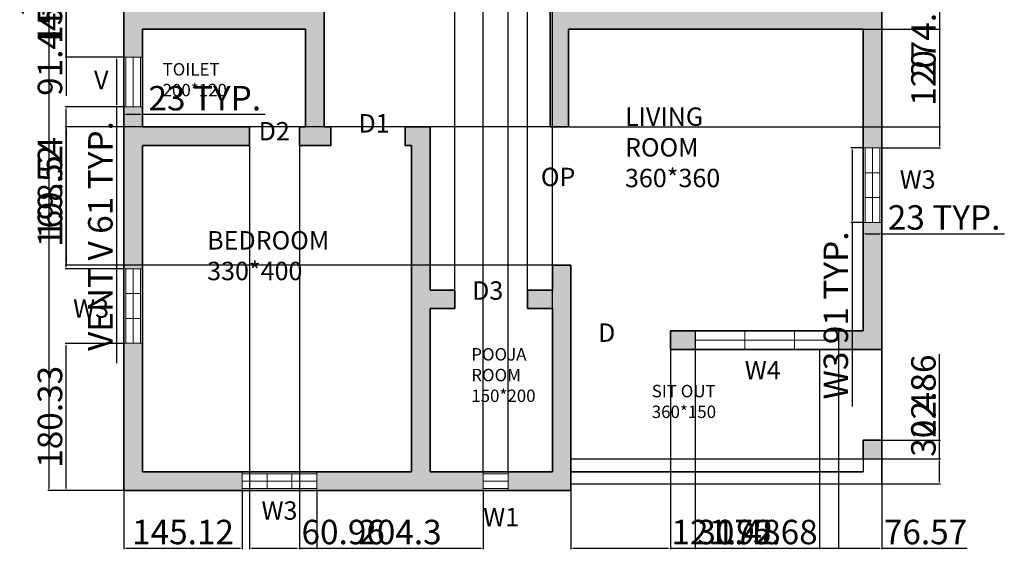
# Model space of a CAD drawing. Units: centimetres. Extents: x 2091 to 3299, y 1401 to 2845.
# Tile 1 of 2: x 2091 to 3299, y 1401 to 2053. Entities that reach past the tile are written whole.
import ezdxf

# ---------------------------------------------------------------- set-up
doc = ezdxf.new("R2010")
doc.units = ezdxf.units.CM
for name, color, linetype, lineweight in [('A-ANNO-DIMS', 2, 'Continuous', 18), ('A-ANNO-TEXT', 7, 'Continuous', 18), ('A-AREA-IDEN', 7, 'Continuous', 25), ('A-FLOR-STRS', 7, 'Continuous', 25), ('A-GLAZ', 4, 'Continuous', 18), ('A-WALL', 7, 'Continuous', 35)]:
    doc.layers.add(name, color=color, linetype=linetype, lineweight=lineweight)
doc.layers.add('A-WALL-PATT', color=18, linetype='Continuous', lineweight=13, true_color=0x000000)
doc.styles.get("Standard").update_dxf_attribs({"font": 'arial.ttf'})
doc.dimstyles.new('ISO-25', dxfattribs={"dimtxt": 30, "dimasz": 2.5, "dimexe": 1.25, "dimexo": 0.625, "dimtad": 1, "dimtxsty": 'Standard', "dimcen": 2.5, "dimadec": 0, "dimazin": 0, "dimtfac": 1, "dimtmove": 0, "dimatfit": 3, "dimfxl": 1, "dimarcsym": 0})

# ---------------------------------------------------------------- blocks, each defined once
blk = doc.blocks.new('*D2')
at = {"layer": 'A-ANNO-DIMS', "color": 0, "lineweight": -2, "transparency": 16777216}
for p, q in [((2218.2, 2725.5), (2125.3, 2725.5)), ((2126.6, 2723), (2126.6, 1478)), ((2218.2, 1475.5), (2125.3, 1475.5))]:
    blk.add_line(p, q, dxfattribs=at)
at = {"layer": 'A-ANNO-DIMS', "color": 0, "transparency": 16777216}
for points in [[(2126.2, 2723), (2127, 2723), (2126.6, 2725.5)], [(2126.2, 1478), (2127, 1478), (2126.6, 1475.5)]]:
    blk.add_solid(points, dxfattribs=at)
at = {"layer": 'Defpoints', "color": 0, "transparency": 16777216}
for p in [(2218.9, 2725.5), (2126.6, 1475.5), (2218.9, 1475.5)]:
    blk.add_point(p, dxfattribs=at)
at = {"layer": 'A-ANNO-DIMS', "color": 0, "transparency": 16777216, "insert": (2110.6, 2100.5), "char_height": 30, "attachment_point": 5, "rotation": 90}
blk.add_mtext('1250', dxfattribs=at)
blk = doc.blocks.new('WIN-W3')
for p, q in [((0, 0), (0, 22.9)), ((0, 20.3), (91.4, 20.3)), ((30.5, 2.5), (30.5, 20.3)), ((61, 2.5), (61, 20.3)), ((91.4, 22.9), (91.4, 0)), ((0, 11.4), (91.4, 11.4)), ((91.4, 2.5), (0, 2.5))]:
    blk.add_line(p, q)
blk = doc.blocks.new('VENT-V')
for p, q in [((0, 0), (0, 22.9)), ((0, 20.3), (61, 20.3)), ((61, 22.9), (61, 0)), ((0, 11.4), (61, 11.4)), ((61, 2.5), (0, 2.5))]:
    blk.add_line(p, q)
blk = doc.blocks.new('*D5')
at = {"layer": 'A-ANNO-DIMS', "color": 0, "lineweight": -2, "transparency": 16777216}
for p, q in [((3125.4, 1895.5), (3111, 1895.5)), ((3112.3, 1893), (3112.3, 1806.5)), ((3125.4, 1804), (3111, 1804)), ((3112.3, 1804), (3112.3, 1578.5))]:
    blk.add_line(p, q, dxfattribs=at)
at = {"layer": 'A-ANNO-DIMS', "color": 0, "transparency": 16777216}
for points in [[(3111.9, 1893), (3112.7, 1893), (3112.3, 1895.5)], [(3111.9, 1806.5), (3112.7, 1806.5), (3112.3, 1804)]]:
    blk.add_solid(points, dxfattribs=at)
at = {"layer": 'Defpoints', "color": 0, "transparency": 16777216}
for p in [(3126, 1895.5), (3112.3, 1804), (3126, 1804)]:
    blk.add_point(p, dxfattribs=at)
at = {"layer": 'A-ANNO-DIMS', "color": 0, "transparency": 16777216, "insert": (3096.3, 1690), "char_height": 30, "attachment_point": 5, "rotation": 90}
blk.add_mtext('W3 91 TYP.', dxfattribs=at)
blk = doc.blocks.new('*D6')
at = {"layer": 'A-ANNO-DIMS', "color": 0, "lineweight": -2, "transparency": 16777216}
for p, q in [((3126, 1803.4), (3126, 1789.1)), ((3148.9, 1803.4), (3148.9, 1789.1)), ((3128.5, 1790.3), (3146.4, 1790.3)), ((3148.9, 1790.3), (3299.2, 1790.3))]:
    blk.add_line(p, q, dxfattribs=at)
at = {"layer": 'A-ANNO-DIMS', "color": 0, "transparency": 16777216}
for points in [[(3128.5, 1790.7), (3128.5, 1789.9), (3126, 1790.3)], [(3146.4, 1790.7), (3146.4, 1789.9), (3148.9, 1790.3)]]:
    blk.add_solid(points, dxfattribs=at)
at = {"layer": 'Defpoints', "color": 0, "transparency": 16777216}
for p in [(3126, 1804), (3148.9, 1804), (3148.9, 1790.3)]:
    blk.add_point(p, dxfattribs=at)
at = {"layer": 'A-ANNO-DIMS', "color": 0, "transparency": 16777216, "insert": (3225.3, 1806.3), "char_height": 30, "attachment_point": 5}
blk.add_mtext('23 TYP.', dxfattribs=at)
blk = doc.blocks.new('*D7')
at = {"layer": 'A-ANNO-DIMS', "color": 0, "lineweight": -2, "transparency": 16777216}
for p, q in [((2218.2, 2006.8), (2208.5, 2006.8)), ((2209.7, 2004.3), (2209.7, 1948.3)), ((2218.2, 1945.8), (2208.5, 1945.8)), ((2209.7, 1945.8), (2209.7, 1631.5))]:
    blk.add_line(p, q, dxfattribs=at)
at = {"layer": 'A-ANNO-DIMS', "color": 0, "transparency": 16777216}
for points in [[(2209.3, 2004.3), (2210.1, 2004.3), (2209.7, 2006.8)], [(2209.3, 1948.3), (2210.1, 1948.3), (2209.7, 1945.8)]]:
    blk.add_solid(points, dxfattribs=at)
at = {"layer": 'Defpoints', "color": 0, "transparency": 16777216}
for p in [(2218.9, 2006.8), (2209.7, 1945.8), (2218.9, 1945.8)]:
    blk.add_point(p, dxfattribs=at)
at = {"layer": 'A-ANNO-DIMS', "color": 0, "transparency": 16777216, "insert": (2193.8, 1787.4), "char_height": 30, "attachment_point": 5, "rotation": 90}
blk.add_mtext('VENT V 61 TYP.', dxfattribs=at)
blk = doc.blocks.new('*D8')
at = {"layer": 'A-ANNO-DIMS', "color": 0, "lineweight": -2, "transparency": 16777216}
for p, q in [((2218.9, 1945.2), (2218.9, 1935.4)), ((2221.4, 1936.7), (2239.2, 1936.7)), ((2241.7, 1945.2), (2241.7, 1935.4)), ((2241.7, 1936.7), (2392, 1936.7))]:
    blk.add_line(p, q, dxfattribs=at)
at = {"layer": 'A-ANNO-DIMS', "color": 0, "transparency": 16777216}
for points in [[(2221.4, 1937.1), (2221.4, 1936.3), (2218.9, 1936.7)], [(2239.2, 1937.1), (2239.2, 1936.3), (2241.7, 1936.7)]]:
    blk.add_solid(points, dxfattribs=at)
at = {"layer": 'Defpoints', "color": 0, "transparency": 16777216}
for p in [(2218.9, 1945.8), (2241.7, 1945.8), (2241.7, 1936.7)]:
    blk.add_point(p, dxfattribs=at)
at = {"layer": 'A-ANNO-DIMS', "color": 0, "transparency": 16777216, "insert": (2318.1, 1952.6), "char_height": 30, "attachment_point": 5}
blk.add_mtext('23 TYP.', dxfattribs=at)
blk = doc.blocks.new('*D11')
at = {"layer": 'A-ANNO-DIMS', "color": 0, "lineweight": -2, "transparency": 16777216}
for p, q in [((2373.1, 1897.7), (2373.1, 1403.4)), ((2434.1, 1897.7), (2434.1, 1403.4)), ((2375.6, 1404.6), (2431.6, 1404.6)), ((2434.1, 1404.6), (2539.2, 1404.6))]:
    blk.add_line(p, q, dxfattribs=at)
at = {"layer": 'A-ANNO-DIMS', "color": 0, "transparency": 16777216}
for points in [[(2375.6, 1405), (2375.6, 1404.2), (2373.1, 1404.6)], [(2431.6, 1405), (2431.6, 1404.2), (2434.1, 1404.6)]]:
    blk.add_solid(points, dxfattribs=at)
at = {"layer": 'Defpoints', "color": 0, "transparency": 16777216}
for p in [(2373.1, 1898.4), (2434.1, 1898.4), (2434.1, 1404.6)]:
    blk.add_point(p, dxfattribs=at)
at = {"layer": 'A-ANNO-DIMS', "color": 0, "transparency": 16777216, "insert": (2487.9, 1420.6), "char_height": 30, "attachment_point": 5}
blk.add_mtext('60.96', dxfattribs=at)
blk = doc.blocks.new('*D12')
at = {"layer": 'A-ANNO-DIMS', "color": 0, "lineweight": -2, "transparency": 16777216}
for p, q in [((2625.1, 1721.9), (2625.1, 2797.7)), ((2627.6, 2796.4), (2711.6, 2796.4)), ((2714.1, 1721.9), (2714.1, 2797.7)), ((2714.1, 2796.4), (2819, 2796.4))]:
    blk.add_line(p, q, dxfattribs=at)
at = {"layer": 'A-ANNO-DIMS', "color": 0, "transparency": 16777216}
for points in [[(2627.6, 2796.8), (2627.6, 2796), (2625.1, 2796.4)], [(2711.6, 2796.8), (2711.6, 2796), (2714.1, 2796.4)]]:
    blk.add_solid(points, dxfattribs=at)
at = {"layer": 'Defpoints', "color": 0, "transparency": 16777216}
for p in [(2714.1, 2796.4), (2625.1, 1721.2), (2714.1, 1721.2)]:
    blk.add_point(p, dxfattribs=at)
at = {"layer": 'A-ANNO-DIMS', "color": 0, "transparency": 16777216, "insert": (2767.8, 2812.4), "char_height": 30, "attachment_point": 5}
blk.add_mtext('89.04', dxfattribs=at)
blk = doc.blocks.new('*D13')
at = {"layer": 'A-ANNO-DIMS', "color": 0, "lineweight": -2, "transparency": 16777216}
for p, q in [((2714.1, 1699), (2714.1, 2797.7)), ((2716.6, 2796.4), (2742.1, 2796.4)), ((2744.6, 1699), (2744.6, 2797.7)), ((2744.6, 2796.4), (2849.6, 2796.4))]:
    blk.add_line(p, q, dxfattribs=at)
at = {"layer": 'A-ANNO-DIMS', "color": 0, "transparency": 16777216}
for points in [[(2716.6, 2796.8), (2716.6, 2796), (2714.1, 2796.4)], [(2742.1, 2796.8), (2742.1, 2796), (2744.6, 2796.4)]]:
    blk.add_solid(points, dxfattribs=at)
at = {"layer": 'Defpoints', "color": 0, "transparency": 16777216}
for p in [(2744.6, 2796.4), (2714.1, 1698.4), (2744.6, 1698.4)]:
    blk.add_point(p, dxfattribs=at)
at = {"layer": 'A-ANNO-DIMS', "color": 0, "transparency": 16777216, "insert": (2798.3, 2812.4), "char_height": 30, "attachment_point": 5}
blk.add_mtext('30.48', dxfattribs=at)
blk = doc.blocks.new('*D14')
at = {"layer": 'A-ANNO-DIMS', "color": 0, "lineweight": -2, "transparency": 16777216}
for p, q in [((2741.1, 1921.2), (2146.7, 1921.2)), ((2148, 1918.7), (2148, 1754.2)), ((2744, 1751.7), (2146.7, 1751.7))]:
    blk.add_line(p, q, dxfattribs=at)
at = {"layer": 'A-ANNO-DIMS', "color": 0, "transparency": 16777216}
for points in [[(2147.5, 1918.7), (2148.4, 1918.7), (2148, 1921.2)], [(2147.5, 1754.2), (2148.4, 1754.2), (2148, 1751.7)]]:
    blk.add_solid(points, dxfattribs=at)
at = {"layer": 'Defpoints', "color": 0, "transparency": 16777216}
for p in [(2741.7, 1921.2), (2148, 1751.7), (2744.6, 1751.7)]:
    blk.add_point(p, dxfattribs=at)
at = {"layer": 'A-ANNO-DIMS', "color": 0, "transparency": 16777216, "insert": (2132, 1836.5), "char_height": 30, "attachment_point": 5, "rotation": 90}
blk.add_mtext('169.52', dxfattribs=at)
blk = doc.blocks.new('*D15')
at = {"layer": 'A-ANNO-DIMS', "color": 0, "lineweight": -2, "transparency": 16777216}
for p, q in [((2765.2, 2041.2), (3221, 2041.2)), ((3219.8, 2038.7), (3219.8, 1923.7)), ((2765.2, 1921.2), (3221, 1921.2))]:
    blk.add_line(p, q, dxfattribs=at)
at = {"layer": 'A-ANNO-DIMS', "color": 0, "transparency": 16777216}
for points in [[(3219.3, 2038.7), (3220.2, 2038.7), (3219.8, 2041.2)], [(3219.3, 1923.7), (3220.2, 1923.7), (3219.8, 1921.2)]]:
    blk.add_solid(points, dxfattribs=at)
at = {"layer": 'Defpoints', "color": 0, "transparency": 16777216}
for p in [(2764.6, 2041.2), (2764.6, 1921.2), (3219.8, 1921.2)]:
    blk.add_point(p, dxfattribs=at)
at = {"layer": 'A-ANNO-DIMS', "color": 0, "transparency": 16777216, "insert": (3203.8, 1981.2), "char_height": 30, "attachment_point": 5, "rotation": 90}
blk.add_mtext('120', dxfattribs=at)
blk = doc.blocks.new('*D16')
at = {"layer": 'A-ANNO-DIMS', "color": 0, "lineweight": -2, "transparency": 16777216}
for p, q in [((2767.4, 1751.1), (2767.4, 1403.4)), ((2889.4, 1670.6), (2889.4, 1403.4)), ((2769.9, 1404.6), (2886.9, 1404.6)), ((2889.4, 1404.6), (3014.5, 1404.6))]:
    blk.add_line(p, q, dxfattribs=at)
at = {"layer": 'A-ANNO-DIMS', "color": 0, "transparency": 16777216}
for points in [[(2769.9, 1405), (2769.9, 1404.2), (2767.4, 1404.6)], [(2886.9, 1405), (2886.9, 1404.2), (2889.4, 1404.6)]]:
    blk.add_solid(points, dxfattribs=at)
at = {"layer": 'Defpoints', "color": 0, "transparency": 16777216}
for p in [(2767.4, 1751.7), (2889.4, 1671.2), (2889.4, 1404.6)]:
    blk.add_point(p, dxfattribs=at)
at = {"layer": 'A-ANNO-DIMS', "color": 0, "transparency": 16777216, "insert": (2953.2, 1420.6), "char_height": 30, "attachment_point": 5}
blk.add_mtext('121.92', dxfattribs=at)
blk = doc.blocks.new('*D17')
at = {"layer": 'A-ANNO-DIMS', "color": 0, "lineweight": -2, "transparency": 16777216}
for p, q in [((2919.8, 1670.6), (2919.8, 1403.4)), ((3095.5, 1670.6), (3095.5, 1403.4)), ((2922.3, 1404.6), (3093, 1404.6))]:
    blk.add_line(p, q, dxfattribs=at)
at = {"layer": 'A-ANNO-DIMS', "color": 0, "transparency": 16777216}
for points in [[(2922.3, 1405), (2922.3, 1404.2), (2919.8, 1404.6)], [(3093, 1405), (3093, 1404.2), (3095.5, 1404.6)]]:
    blk.add_solid(points, dxfattribs=at)
at = {"layer": 'Defpoints', "color": 0, "transparency": 16777216}
for p in [(2919.8, 1671.2), (3095.5, 1671.2), (3095.5, 1404.6)]:
    blk.add_point(p, dxfattribs=at)
at = {"layer": 'A-ANNO-DIMS', "color": 0, "transparency": 16777216, "insert": (3007.7, 1420.6), "char_height": 30, "attachment_point": 5}
blk.add_mtext('175.68', dxfattribs=at)
blk = doc.blocks.new('*D18')
at = {"layer": 'A-ANNO-DIMS', "color": 0, "lineweight": -2, "transparency": 16777216}
for p, q in [((2889.4, 1647.7), (2889.4, 1403.4)), ((2919.8, 1647.7), (2919.8, 1403.4)), ((2891.9, 1404.6), (2917.3, 1404.6)), ((2919.8, 1404.6), (3024.9, 1404.6))]:
    blk.add_line(p, q, dxfattribs=at)
at = {"layer": 'A-ANNO-DIMS', "color": 0, "transparency": 16777216}
for points in [[(2891.9, 1405), (2891.9, 1404.2), (2889.4, 1404.6)], [(2917.3, 1405), (2917.3, 1404.2), (2919.8, 1404.6)]]:
    blk.add_solid(points, dxfattribs=at)
at = {"layer": 'Defpoints', "color": 0, "transparency": 16777216}
for p in [(2889.4, 1648.4), (2919.8, 1648.4), (2919.8, 1404.6)]:
    blk.add_point(p, dxfattribs=at)
at = {"layer": 'A-ANNO-DIMS', "color": 0, "transparency": 16777216, "insert": (2973.6, 1420.6), "char_height": 30, "attachment_point": 5}
blk.add_mtext('30.48', dxfattribs=at)
blk = doc.blocks.new('*D21')
at = {"layer": 'A-ANNO-DIMS', "color": 0, "lineweight": -2, "transparency": 16777216}
for p, q in [((2241.1, 2155.5), (2146.7, 2155.5)), ((2148, 2153), (2148, 2066.6)), ((2241.1, 2064.1), (2146.7, 2064.1)), ((2148, 2064.1), (2148, 1959.2))]:
    blk.add_line(p, q, dxfattribs=at)
at = {"layer": 'A-ANNO-DIMS', "color": 0, "transparency": 16777216}
for points in [[(2147.5, 2153), (2148.4, 2153), (2148, 2155.5)], [(2147.5, 2066.6), (2148.4, 2066.6), (2148, 2064.1)]]:
    blk.add_solid(points, dxfattribs=at)
at = {"layer": 'Defpoints', "color": 0, "transparency": 16777216}
for p in [(2241.7, 2155.5), (2148, 2064.1), (2241.7, 2064.1)]:
    blk.add_point(p, dxfattribs=at)
at = {"layer": 'A-ANNO-DIMS', "color": 0, "transparency": 16777216, "insert": (2132, 2010.4), "char_height": 30, "attachment_point": 5, "rotation": 90}
blk.add_mtext('91.44', dxfattribs=at)
blk = doc.blocks.new('*D22')
at = {"layer": 'A-ANNO-DIMS', "color": 0, "lineweight": -2, "transparency": 16777216}
for p, q in [((2218.9, 1474.9), (2218.9, 1403.4)), ((2364, 1474.9), (2364, 1403.4)), ((2221.4, 1404.6), (2361.5, 1404.6))]:
    blk.add_line(p, q, dxfattribs=at)
at = {"layer": 'A-ANNO-DIMS', "color": 0, "transparency": 16777216}
for points in [[(2221.4, 1405), (2221.4, 1404.2), (2218.9, 1404.6)], [(2361.5, 1405), (2361.5, 1404.2), (2364, 1404.6)]]:
    blk.add_solid(points, dxfattribs=at)
at = {"layer": 'Defpoints', "color": 0, "transparency": 16777216}
for p in [(2218.9, 1475.5), (2364, 1475.5), (2364, 1404.6)]:
    blk.add_point(p, dxfattribs=at)
at = {"layer": 'A-ANNO-DIMS', "color": 0, "transparency": 16777216, "insert": (2291.4, 1420.6), "char_height": 30, "attachment_point": 5}
blk.add_mtext('145.12', dxfattribs=at)
blk = doc.blocks.new('*D23')
at = {"layer": 'A-ANNO-DIMS', "color": 0, "lineweight": -2, "transparency": 16777216}
for p, q in [((2455.4, 1474.9), (2455.4, 1403.4)), ((2659.7, 1474.9), (2659.7, 1403.4)), ((2457.9, 1404.6), (2657.2, 1404.6))]:
    blk.add_line(p, q, dxfattribs=at)
at = {"layer": 'A-ANNO-DIMS', "color": 0, "transparency": 16777216}
for points in [[(2457.9, 1405), (2457.9, 1404.2), (2455.4, 1404.6)], [(2657.2, 1405), (2657.2, 1404.2), (2659.7, 1404.6)]]:
    blk.add_solid(points, dxfattribs=at)
at = {"layer": 'Defpoints', "color": 0, "transparency": 16777216}
for p in [(2455.4, 1475.5), (2659.7, 1475.5), (2659.7, 1404.6)]:
    blk.add_point(p, dxfattribs=at)
at = {"layer": 'A-ANNO-DIMS', "color": 0, "transparency": 16777216, "insert": (2557.6, 1420.6), "char_height": 30, "attachment_point": 5}
blk.add_mtext('204.3', dxfattribs=at)
blk = doc.blocks.new('*D24')
at = {"layer": 'A-ANNO-DIMS', "color": 0, "lineweight": -2, "transparency": 16777216}
for p, q in [((2659.7, 1499), (2659.7, 2797.7)), ((2662.2, 2796.4), (2687.7, 2796.4)), ((2690.2, 1499), (2690.2, 2797.7)), ((2690.2, 2796.4), (2795.2, 2796.4))]:
    blk.add_line(p, q, dxfattribs=at)
at = {"layer": 'A-ANNO-DIMS', "color": 0, "transparency": 16777216}
for points in [[(2662.2, 2796.8), (2662.2, 2796), (2659.7, 2796.4)], [(2687.7, 2796.8), (2687.7, 2796), (2690.2, 2796.4)]]:
    blk.add_solid(points, dxfattribs=at)
at = {"layer": 'Defpoints', "color": 0, "transparency": 16777216}
for p in [(2690.2, 2796.4), (2659.7, 1498.4), (2690.2, 1498.4)]:
    blk.add_point(p, dxfattribs=at)
at = {"layer": 'A-ANNO-DIMS', "color": 0, "transparency": 16777216, "insert": (2744, 2812.4), "char_height": 30, "attachment_point": 5}
blk.add_mtext('30.48', dxfattribs=at)
blk = doc.blocks.new('*D25')
at = {"layer": 'A-ANNO-DIMS', "color": 0, "lineweight": -2, "transparency": 16777216}
for p, q in [((2218.2, 1655.8), (2146.7, 1655.8)), ((2148, 1478), (2148, 1653.3)), ((2218.2, 1475.5), (2146.7, 1475.5))]:
    blk.add_line(p, q, dxfattribs=at)
at = {"layer": 'A-ANNO-DIMS', "color": 0, "transparency": 16777216}
for points in [[(2147.5, 1653.3), (2148.4, 1653.3), (2148, 1655.8)], [(2147.5, 1478), (2148.4, 1478), (2148, 1475.5)]]:
    blk.add_solid(points, dxfattribs=at)
at = {"layer": 'Defpoints', "color": 0, "transparency": 16777216}
for p in [(2148, 1655.8), (2218.9, 1655.8), (2218.9, 1475.5)]:
    blk.add_point(p, dxfattribs=at)
at = {"layer": 'A-ANNO-DIMS', "color": 0, "transparency": 16777216, "insert": (2132, 1565.7), "char_height": 30, "attachment_point": 5, "rotation": 90}
blk.add_mtext('180.33', dxfattribs=at)
blk = doc.blocks.new('*D26')
at = {"layer": 'A-ANNO-DIMS', "color": 0, "lineweight": -2, "transparency": 16777216}
for p, q in [((2218.2, 1945.8), (2146.7, 1945.8)), ((2148, 1749.8), (2148, 1943.3)), ((2218.2, 1747.3), (2146.7, 1747.3))]:
    blk.add_line(p, q, dxfattribs=at)
at = {"layer": 'A-ANNO-DIMS', "color": 0, "transparency": 16777216}
for points in [[(2147.5, 1943.3), (2148.4, 1943.3), (2148, 1945.8)], [(2147.5, 1749.8), (2148.4, 1749.8), (2148, 1747.3)]]:
    blk.add_solid(points, dxfattribs=at)
at = {"layer": 'Defpoints', "color": 0, "transparency": 16777216}
for p in [(2148, 1945.8), (2218.9, 1945.8), (2218.9, 1747.3)]:
    blk.add_point(p, dxfattribs=at)
at = {"layer": 'A-ANNO-DIMS', "color": 0, "transparency": 16777216, "insert": (2132, 1846.6), "char_height": 30, "attachment_point": 5, "rotation": 90}
blk.add_mtext('198.54', dxfattribs=at)
blk = doc.blocks.new('*D27')
at = {"layer": 'A-ANNO-DIMS', "color": 0, "lineweight": -2, "transparency": 16777216}
for p, q in [((2218.2, 2164.2), (2146.7, 2164.2)), ((2148, 2009.3), (2148, 2161.7)), ((2218.2, 2006.8), (2146.7, 2006.8))]:
    blk.add_line(p, q, dxfattribs=at)
at = {"layer": 'A-ANNO-DIMS', "color": 0, "transparency": 16777216}
for points in [[(2147.5, 2161.7), (2148.4, 2161.7), (2148, 2164.2)], [(2147.5, 2009.3), (2148.4, 2009.3), (2148, 2006.8)]]:
    blk.add_solid(points, dxfattribs=at)
at = {"layer": 'Defpoints', "color": 0, "transparency": 16777216}
for p in [(2148, 2164.2), (2218.9, 2164.2), (2218.9, 2006.8)]:
    blk.add_point(p, dxfattribs=at)
at = {"layer": 'A-ANNO-DIMS', "color": 0, "transparency": 16777216, "insert": (2132, 2085.5), "char_height": 30, "attachment_point": 5, "rotation": 90}
blk.add_mtext('157.44', dxfattribs=at)
blk = doc.blocks.new('*D33')
at = {"layer": 'A-ANNO-DIMS', "color": 0, "lineweight": -2, "transparency": 16777216}
for p, q in [((3149.5, 2169.8), (3221, 2169.8)), ((3219.8, 2167.3), (3219.8, 1898)), ((3149.5, 1895.5), (3221, 1895.5))]:
    blk.add_line(p, q, dxfattribs=at)
at = {"layer": 'A-ANNO-DIMS', "color": 0, "transparency": 16777216}
for points in [[(3219.3, 2167.3), (3220.2, 2167.3), (3219.8, 2169.8)], [(3219.3, 1898), (3220.2, 1898), (3219.8, 1895.5)]]:
    blk.add_solid(points, dxfattribs=at)
at = {"layer": 'Defpoints', "color": 0, "transparency": 16777216}
for p in [(3148.9, 2169.8), (3148.9, 1895.5), (3219.8, 1895.5)]:
    blk.add_point(p, dxfattribs=at)
at = {"layer": 'A-ANNO-DIMS', "color": 0, "transparency": 16777216, "insert": (3203.8, 2032.6), "char_height": 30, "attachment_point": 5, "rotation": 90}
blk.add_mtext('274.3', dxfattribs=at)
blk = doc.blocks.new('*D34')
at = {"layer": 'A-ANNO-DIMS', "color": 0, "lineweight": -2, "transparency": 16777216}
for p, q in [((3072.3, 1513.5), (3072.3, 1403.4)), ((3148.9, 1513.5), (3148.9, 1403.4)), ((3074.8, 1404.6), (3146.4, 1404.6)), ((3148.9, 1404.6), (3253.6, 1404.6))]:
    blk.add_line(p, q, dxfattribs=at)
at = {"layer": 'A-ANNO-DIMS', "color": 0, "transparency": 16777216}
for points in [[(3074.8, 1405), (3074.8, 1404.2), (3072.3, 1404.6)], [(3146.4, 1405), (3146.4, 1404.2), (3148.9, 1404.6)]]:
    blk.add_solid(points, dxfattribs=at)
at = {"layer": 'Defpoints', "color": 0, "transparency": 16777216}
for p in [(3072.3, 1514.1), (3148.9, 1514.1), (3148.9, 1404.6)]:
    blk.add_point(p, dxfattribs=at)
at = {"layer": 'A-ANNO-DIMS', "color": 0, "transparency": 16777216, "insert": (3202.5, 1420.6), "char_height": 30, "attachment_point": 5}
blk.add_mtext('76.57', dxfattribs=at)
blk = doc.blocks.new('*D35')
at = {"layer": 'A-ANNO-DIMS', "color": 0, "lineweight": -2, "transparency": 16777216}
for p, q in [((3219.8, 1514.1), (3219.8, 1619.1)), ((3149.5, 1514.1), (3221, 1514.1)), ((3219.8, 1486.1), (3219.8, 1511.6)), ((3149.5, 1483.6), (3221, 1483.6))]:
    blk.add_line(p, q, dxfattribs=at)
at = {"layer": 'A-ANNO-DIMS', "color": 0, "transparency": 16777216}
for points in [[(3219.3, 1511.6), (3220.2, 1511.6), (3219.8, 1514.1)], [(3219.3, 1486.1), (3220.2, 1486.1), (3219.8, 1483.6)]]:
    blk.add_solid(points, dxfattribs=at)
at = {"layer": 'Defpoints', "color": 0, "transparency": 16777216}
for p in [(3148.9, 1514.1), (3219.8, 1514.1), (3148.9, 1483.6)]:
    blk.add_point(p, dxfattribs=at)
at = {"layer": 'A-ANNO-DIMS', "color": 0, "transparency": 16777216, "insert": (3203.8, 1567.9), "char_height": 30, "attachment_point": 5, "rotation": 90}
blk.add_mtext('30.48', dxfattribs=at)
blk = doc.blocks.new('*D36')
at = {"layer": 'A-ANNO-DIMS', "color": 0, "lineweight": -2, "transparency": 16777216}
for p, q in [((3219.8, 1537), (3219.8, 1642.4)), ((3149.5, 1537), (3221, 1537)), ((3219.8, 1516.6), (3219.8, 1534.5)), ((3149.5, 1514.1), (3221, 1514.1))]:
    blk.add_line(p, q, dxfattribs=at)
at = {"layer": 'A-ANNO-DIMS', "color": 0, "transparency": 16777216}
for points in [[(3219.3, 1534.5), (3220.2, 1534.5), (3219.8, 1537)], [(3219.3, 1516.6), (3220.2, 1516.6), (3219.8, 1514.1)]]:
    blk.add_solid(points, dxfattribs=at)
at = {"layer": 'Defpoints', "color": 0, "transparency": 16777216}
for p in [(3148.9, 1537), (3219.8, 1537), (3148.9, 1514.1)]:
    blk.add_point(p, dxfattribs=at)
at = {"layer": 'A-ANNO-DIMS', "color": 0, "transparency": 16777216, "insert": (3203.8, 1591), "char_height": 30, "attachment_point": 5, "rotation": 90}
blk.add_mtext('22.86', dxfattribs=at)

msp = doc.modelspace()

# ---------------------------------------------------------------- hatches: boundary and pattern name
at = {"layer": 'A-WALL-PATT'}
h = msp.add_hatch(color=256, dxfattribs=at)
h.dxf.hatch_style = 1
h.paths.add_polyline_path([(2629.919, 2725.51), (2218.865, 2725.51), (2218.865, 2614.708), (2241.725, 2614.708), (2241.725, 2702.65), (2571.725, 2702.65), (2571.725, 2695.03), (2594.585, 2695.03), (2594.585, 2702.65), (2629.919, 2702.65)])
h.paths.add_polyline_path([(2902.29, 2725.51), (2690.879, 2725.51), (2690.879, 2702.65), (2714.585, 2702.65), (2714.585, 2522.65), (2594.585, 2522.65), (2594.585, 2634.77), (2571.725, 2634.77), (2571.725, 2386.95), (2564.105, 2386.95), (2564.105, 2364.09), (2602.205, 2364.09), (2602.205, 2386.95), (2594.585, 2386.95), (2594.585, 2499.79), (2737.445, 2499.79), (2737.445, 2702.65), (2902.29, 2702.65)])
h.paths.add_polyline_path([(3148.865, 2725.51), (2993.73, 2725.51), (2993.73, 2702.65), (3126.005, 2702.65), (3126.005, 2600.88), (3148.865, 2600.88)])
h.paths.add_polyline_path([(3148.865, 2509.44), (3126.005, 2509.44), (3126.005, 2386.95), (2693.645, 2386.95), (2693.645, 2364.09), (2741.725, 2364.09), (2741.725, 2356.47), (2764.585, 2356.47), (2764.585, 2364.09), (3126.005, 2364.09), (3126.005, 2261.228), (3148.865, 2261.228)])
h.paths.add_polyline_path([(2472.665, 2386.95), (2241.725, 2386.95), (2241.725, 2523.268), (2218.865, 2523.268), (2218.865, 2255.666), (2241.725, 2255.666), (2241.725, 2364.09), (2472.665, 2364.09)])
h.paths.add_polyline_path([(3148.865, 2169.788), (3126.005, 2169.788), (3126.005, 2064.09), (2764.585, 2064.09), (2764.585, 2265.03), (2741.725, 2265.03), (2741.725, 1921.23), (2764.585, 1921.23), (2764.585, 2041.23), (3126.005, 2041.23), (3126.005, 1895.472), (3148.865, 1895.472)])
h.paths.add_polyline_path([(3148.865, 1804.032), (3126.005, 1804.032), (3126.005, 1671.23), (3095.525, 1671.23), (3095.525, 1648.37), (3148.865, 1648.37)])
h.paths.add_polyline_path([(2241.725, 2155.53), (2241.725, 2164.226), (2218.865, 2164.226), (2218.865, 2006.784), (2241.725, 2006.784), (2241.725, 2041.23), (2441.725, 2041.23), (2441.725, 1921.23), (2434.105, 1921.23), (2434.105, 1898.37), (2472.665, 1898.37), (2472.665, 1921.23), (2464.585, 1921.23), (2464.585, 2064.09), (2241.725, 2064.09)])
h.paths.add_polyline_path([(2241.725, 1898.37), (2373.145, 1898.37), (2373.145, 1921.23), (2241.725, 1921.23), (2241.725, 1945.824), (2218.865, 1945.824), (2218.865, 1747.285), (2241.725, 1747.285)])
h.paths.add_polyline_path([(2241.725, 1655.845), (2218.865, 1655.845), (2218.865, 1475.51), (2363.981, 1475.51), (2363.981, 1498.37), (2241.725, 1498.37)])
h.paths.add_polyline_path([(2594.585, 1921.23), (2564.105, 1921.23), (2564.105, 1898.37), (2571.725, 1898.37), (2571.725, 1498.37), (2455.421, 1498.37), (2455.421, 1475.51), (2659.718, 1475.51), (2659.718, 1498.37), (2594.585, 1498.37), (2594.585, 1698.37), (2625.065, 1698.37), (2625.065, 1721.23), (2594.585, 1721.23)])
h.paths.add_polyline_path([(2767.445, 1721.23), (2767.445, 1751.71), (2744.585, 1751.71), (2744.585, 1721.23), (2714.105, 1721.23), (2714.105, 1698.37), (2744.585, 1698.37), (2744.585, 1498.37), (2690.198, 1498.37), (2690.198, 1475.51), (2767.445, 1475.51)])
h.paths.add_polyline_path([(3148.865, 1536.968), (3126.005, 1536.968), (3126.005, 1514.108), (3148.865, 1514.108)])
h.paths.add_polyline_path([(2919.845, 1671.23), (2889.365, 1671.23), (2889.365, 1648.37), (2919.845, 1648.37)])

# ---------------------------------------------------------------- linework, layer by layer
at = {"layer": 'A-FLOR-STRS'}
for p, q in [((3072.296, 1648.37), (3072.296, 1514.108)), ((2767.445, 1514.108), (3148.865, 1514.108)), ((3126.005, 1514.108), (3126.005, 1498.37)), ((3126.005, 1498.37), (2767.445, 1498.37)), ((2767.445, 1498.37), (3126.005, 1498.37)), ((2767.445, 1483.628), (3148.865, 1483.628))]:
    msp.add_line(p, q, dxfattribs=at)
at = {"layer": 'A-GLAZ'}
for p, q in [((2919.845, 1648.37), (2919.845, 1671.23)), ((2980.805, 1648.37), (2980.805, 1671.23)), ((3041.765, 1648.37), (3041.765, 1671.23)), ((3095.525, 1671.23), (3095.525, 1648.37)), ((2919.845, 1659.8), (3095.525, 1659.8)), ((2659.718, 1498.37), (2659.718, 1475.51)), ((2690.198, 1475.51), (2690.198, 1498.37)), ((2690.198, 1495.83), (2659.718, 1495.83)), ((2659.718, 1486.94), (2690.198, 1486.94)), ((2659.718, 1478.05), (2690.198, 1478.05))]:
    msp.add_line(p, q, dxfattribs=at)
at = {"layer": 'A-WALL'}
for p, q in [((2218.865, 1475.51), (2218.865, 2725.51)), ((3148.865, 2725.51), (3148.865, 1483.628)), ((2741.725, 1921.23), (2741.725, 2265.03)), ((2464.585, 2064.09), (2464.585, 1921.23)), ((2441.725, 2041.23), (2241.725, 2041.23)), ((2241.725, 1921.23), (2241.725, 2041.23)), ((2441.725, 2041.23), (2441.725, 1921.23)), ((3126.005, 2041.23), (2764.585, 2041.23)), ((2764.585, 1921.23), (2764.585, 2041.23)), ((3126.005, 2041.23), (3126.005, 1671.23)), ((2373.145, 1921.23), (2241.725, 1921.23)), ((2373.145, 1921.23), (2373.145, 1898.37)), ((2434.105, 1921.23), (2434.105, 1898.37)), ((2441.725, 1921.23), (2434.105, 1921.23)), ((2472.665, 1921.23), (2464.585, 1921.23)), ((2472.665, 1898.37), (2472.665, 1921.23)), ((2564.105, 1898.37), (2564.105, 1921.23)), ((2594.585, 1921.23), (2564.105, 1921.23)), ((2594.585, 1721.23), (2594.585, 1921.23)), ((2741.725, 1921.23), (2764.585, 1921.23)), ((2241.725, 1498.37), (2241.725, 1898.37)), ((2373.145, 1898.37), (2241.725, 1898.37)), ((2472.665, 1898.37), (2434.105, 1898.37)), ((2571.725, 1898.37), (2564.105, 1898.37)), ((2571.725, 1498.37), (2571.725, 1898.37)), ((2767.445, 1751.71), (2744.585, 1751.71)), ((2744.585, 1751.71), (2744.585, 1721.23)), ((2767.445, 1721.23), (2767.445, 1751.71)), ((2594.585, 1721.23), (2625.065, 1721.23)), ((2625.065, 1698.37), (2625.065, 1721.23)), ((2714.105, 1698.37), (2714.105, 1721.23)), ((2714.105, 1721.23), (2744.585, 1721.23)), ((2767.445, 1475.51), (2767.445, 1721.23)), ((2594.585, 1498.37), (2594.585, 1698.37)), ((2594.585, 1698.37), (2625.065, 1698.37)), ((2594.585, 1698.37), (2625.065, 1698.37)), ((2594.585, 1698.37), (2625.065, 1698.37)), ((2714.105, 1698.37), (2744.585, 1698.37)), ((2744.585, 1698.37), (2741.105, 1698.37)), ((2744.585, 1498.37), (2744.585, 1698.37)), ((2889.365, 1671.23), (3126.005, 1671.23)), ((2889.365, 1648.37), (2889.365, 1671.23)), ((2889.365, 1648.37), (3148.865, 1648.37)), ((3126.005, 1514.108), (3126.005, 1536.968)), ((3126.005, 1536.968), (3148.865, 1536.968)), ((2571.725, 1498.37), (2241.725, 1498.37)), ((2744.585, 1498.37), (2594.585, 1498.37)), ((2767.445, 1475.51), (2218.865, 1475.51))]:
    msp.add_line(p, q, dxfattribs=at)

# ---------------------------------------------------------------- block references
at = {"layer": 'A-GLAZ'}
for name, p, rotation in [('VENT-V', (2218.866, 2006.784), 269.9999999999984), ('WIN-W3', (3126.006, 1895.472), 270), ('WIN-W3', (2218.866, 1747.285), 270.0000000000006)]:
    msp.add_blockref(name, p, dxfattribs=dict(at, rotation=rotation))
msp.add_blockref('WIN-W3', (2363.981, 1475.51), dxfattribs=at)

# ---------------------------------------------------------------- texts
at = {"layer": 'A-ANNO-TEXT', "char_height": 22.56, "attachment_point": 1}
for s, width, insert in [('V', 39.89904, (2182.186, 1989.998)), ('D1', 21.81012, (2506.661, 1936.92)), ('D2', 22.59147, (2384.165, 1927.249)), ('OP', 36.39872, (2730.479, 1871.174)), ('W3', 162.65151, (3170.799, 1868.053)), ('D3', 40.55497, (2646.093, 1731.861)), ('W3', 162.65151, (2156.466, 1709.852)), ('D', 51.99818, (2800.676, 1680.233)), ('W4', 162.65151, (2980.628, 1634.308)), ('W3', 162.65151, (2387.643, 1462.118)), ('W1', 162.65151, (2659.718, 1454.126))]:
    msp.add_mtext_dynamic_manual_height_columns(s, width=width, gutter_width=12.5, heights=[0], dxfattribs=dict(at, insert=insert))
at = {"layer": 'A-AREA-IDEN', "attachment_point": 1}
for s, width, insert, char_height in [('TOILET\\P200*120', 85.88212, (2266.279, 1999.409), 15.24), ('LIVING ROOM\\P360*360', 166.11333, (2833.712, 1945.065), 22.56), ('BEDROOM\\P330*400', 184.57037, (2321.017, 1793.427), 22.56), ('POOJA ROOM \\P150*200', 65.62503, (2645.04, 1649.986), 15.24), ('SIT OUT \\P360*150', 92.28519, (2866.525, 1604.905), 15.24)]:
    msp.add_mtext_dynamic_manual_height_columns(s, width=width, gutter_width=12.5, heights=[0], dxfattribs=dict(at, insert=insert, char_height=char_height))

# ---------------------------------------------------------------- dimensions: what is measured, and where the dimension line sits
at = {"layer": 'A-ANNO-DIMS'}
for base, p1, p2, override, picture, middle in [((2714.105, 2796.41), (2625.065, 1721.23), (2714.105, 1721.23), {"dimdec": 2, "dimlfac": 1, "dimrnd": 0, "dimzin": 0, "dimdsep": 46, "dimlunit": 2}, '*D12', (2767.807, 2812.352)), ((2690.198, 2796.41), (2659.718, 1498.37), (2690.198, 1498.37), {"dimdec": 2, "dimlfac": 1, "dimrnd": 0, "dimzin": 0, "dimdsep": 46, "dimlunit": 2}, '*D24', (2743.961, 2812.362)), ((2744.585, 2796.41), (2714.105, 1698.37), (2744.585, 1698.37), {"dimdec": 2, "dimlfac": 1, "dimrnd": 0, "dimzin": 0, "dimdsep": 46, "dimlunit": 2}, '*D13', (2798.348, 2812.362)), ((2434.105, 1404.61), (2373.145, 1898.37), (2434.105, 1898.37), {"dimdec": 2, "dimlfac": 1, "dimrnd": 0, "dimzin": 0, "dimdsep": 46, "dimlunit": 2}, '*D11', (2487.919, 1420.552)), ((2889.365, 1404.61), (2767.445, 1751.71), (2889.365, 1671.23), {"dimdec": 2, "dimlfac": 1, "dimrnd": 0, "dimzin": 0, "dimdsep": 46, "dimlunit": 2}, '*D16', (2953.196, 1420.552)), ((3095.525, 1404.61), (2919.845, 1671.23), (3095.525, 1671.23), {"dimdec": 2, "dimlfac": 1, "dimrnd": 0, "dimzin": 0, "dimdsep": 46, "dimlunit": 2}, '*D17', (3007.685, 1420.552)), ((2919.845, 1404.61), (2889.365, 1648.37), (2919.845, 1648.37), {"dimdec": 2, "dimlfac": 1, "dimrnd": 0, "dimzin": 0, "dimdsep": 46, "dimlunit": 2}, '*D18', (2973.608, 1420.562)), ((3148.865, 1404.61), (3072.296, 1514.108), (3148.865, 1514.108), {"dimdec": 2, "dimlfac": 1, "dimrnd": 0, "dimzin": 0, "dimdsep": 46, "dimlunit": 2}, '*D34', (3202.485, 1420.552)), ((2363.981, 1404.61), (2218.865, 1475.51), (2363.981, 1475.51), {"dimdec": 2, "dimlfac": 1, "dimrnd": 0, "dimzin": 0, "dimdsep": 46, "dimlunit": 2}, '*D22', (2291.423, 1420.552)), ((2659.718, 1404.61), (2455.421, 1475.51), (2659.718, 1475.51), {"dimdec": 1, "dimlfac": 1, "dimrnd": 0, "dimzin": 0, "dimdsep": 46, "dimlunit": 2}, '*D23', (2557.57, 1420.562))]:
    dim = msp.add_linear_dim(base=base, p1=p1, p2=p2, dimstyle='ISO-25', override=override, dxfattribs=at)
    dim.commit()
    dim.dimension.update_dxf_attribs({"geometry": picture, "text_midpoint": middle})
for base, p1, p2, override, picture, middle in [((2126.587, 1475.51), (2218.865, 2725.51), (2218.865, 1475.51), {"dimclrd": 0, "dimclre": 0, "dimclrt": 0}, '*D2', (2110.644, 2100.51)), ((2147.965, 2164.226), (2218.865, 2006.784), (2218.865, 2164.226), {"dimdec": 2, "dimlfac": 1, "dimrnd": 0, "dimzin": 0, "dimdsep": 46, "dimlunit": 2}, '*D27', (2132.023, 2085.505)), ((3219.765, 1895.472), (3148.865, 2169.788), (3148.865, 1895.472), {"dimdec": 1, "dimlfac": 1, "dimrnd": 0, "dimzin": 0, "dimdsep": 46, "dimlunit": 2}, '*D33', (3203.813, 2032.63)), ((2147.965, 2064.09), (2241.725, 2155.53), (2241.725, 2064.09), {"dimdec": 2, "dimlfac": 1, "dimrnd": 0, "dimzin": 0, "dimdsep": 46, "dimlunit": 2}, '*D21', (2132.023, 2010.409)), ((3219.765, 1921.23), (2764.585, 2041.23), (2764.585, 1921.23), {"dimdec": 0, "dimlfac": 1, "dimrnd": 0, "dimzin": 0, "dimdsep": 46, "dimlunit": 2}, '*D15', (3203.823, 1981.23)), ((2147.965, 1945.824), (2218.865, 1747.285), (2218.865, 1945.824), {"dimdec": 2, "dimlfac": 1, "dimrnd": 0, "dimzin": 0, "dimdsep": 46, "dimlunit": 2}, '*D26', (2132.023, 1846.554)), ((2147.965, 1751.71), (2741.725, 1921.23), (2744.585, 1751.71), {"dimdec": 2, "dimlfac": 1, "dimrnd": 0, "dimzin": 0, "dimdsep": 46, "dimlunit": 2}, '*D14', (2132.023, 1836.47)), ((2147.96546, 1655.84487), (2218.86546, 1475.50989), (2218.86546, 1655.84487), {"dimdec": 2, "dimlfac": 1, "dimrnd": 0, "dimzin": 0, "dimdsep": 46, "dimlunit": 2}, '*D25', (2132.01304, 1565.67738)), ((3219.765, 1536.968), (3148.865, 1514.108), (3148.865, 1536.968), {"dimdec": 2, "dimlfac": 1, "dimrnd": 0, "dimzin": 0, "dimdsep": 46, "dimlunit": 2}, '*D36', (3203.823, 1590.956)), ((3219.765, 1514.108), (3148.865, 1483.628), (3148.865, 1514.108), {"dimdec": 2, "dimlfac": 1, "dimrnd": 0, "dimzin": 0, "dimdsep": 46, "dimlunit": 2}, '*D35', (3203.813, 1567.871))]:
    dim = msp.add_linear_dim(base=base, p1=p1, p2=p2, angle=90, dimstyle='ISO-25', override=override, dxfattribs=at)
    dim.commit()
    dim.dimension.update_dxf_attribs({"geometry": picture, "text_midpoint": middle})
for base, p1, p2, text, picture, middle in [((2209.721, 1945.824), (2218.865, 2006.784), (2218.865, 1945.824), 'VENT V <> TYP.', '*D7', (2193.779, 1787.399)), ((3112.289, 1804.032), (3126.005, 1895.472), (3126.005, 1804.032), 'W3 <> TYP.', '*D5', (3096.337, 1690.024))]:
    dim = msp.add_linear_dim(base=base, p1=p1, p2=p2, angle=270, text=text, dimstyle='ISO-25', override={"dimdec": 0, "dimlfac": 1, "dimrnd": 0, "dimzin": 0, "dimdsep": 46, "dimlunit": 2}, dxfattribs=at)
    dim.commit()
    dim.dimension.update_dxf_attribs({"geometry": picture, "text_midpoint": middle})
for base, p1, p2, picture, middle in [((2241.725, 1936.68), (2218.865, 1945.824), (2241.725, 1945.824), '*D8', (2318.121, 1952.632)), ((3148.865, 1790.316), (3126.005, 1804.032), (3148.865, 1804.032), '*D6', (3225.261, 1806.268))]:
    dim = msp.add_linear_dim(base=base, p1=p1, p2=p2, text='<> TYP.', dimstyle='ISO-25', override={"dimdec": 0, "dimlfac": 1, "dimrnd": 0, "dimzin": 0, "dimdsep": 46, "dimlunit": 2}, dxfattribs=at)
    dim.commit()
    dim.dimension.update_dxf_attribs({"geometry": picture, "text_midpoint": middle})

doc.saveas('drawing.dxf')
